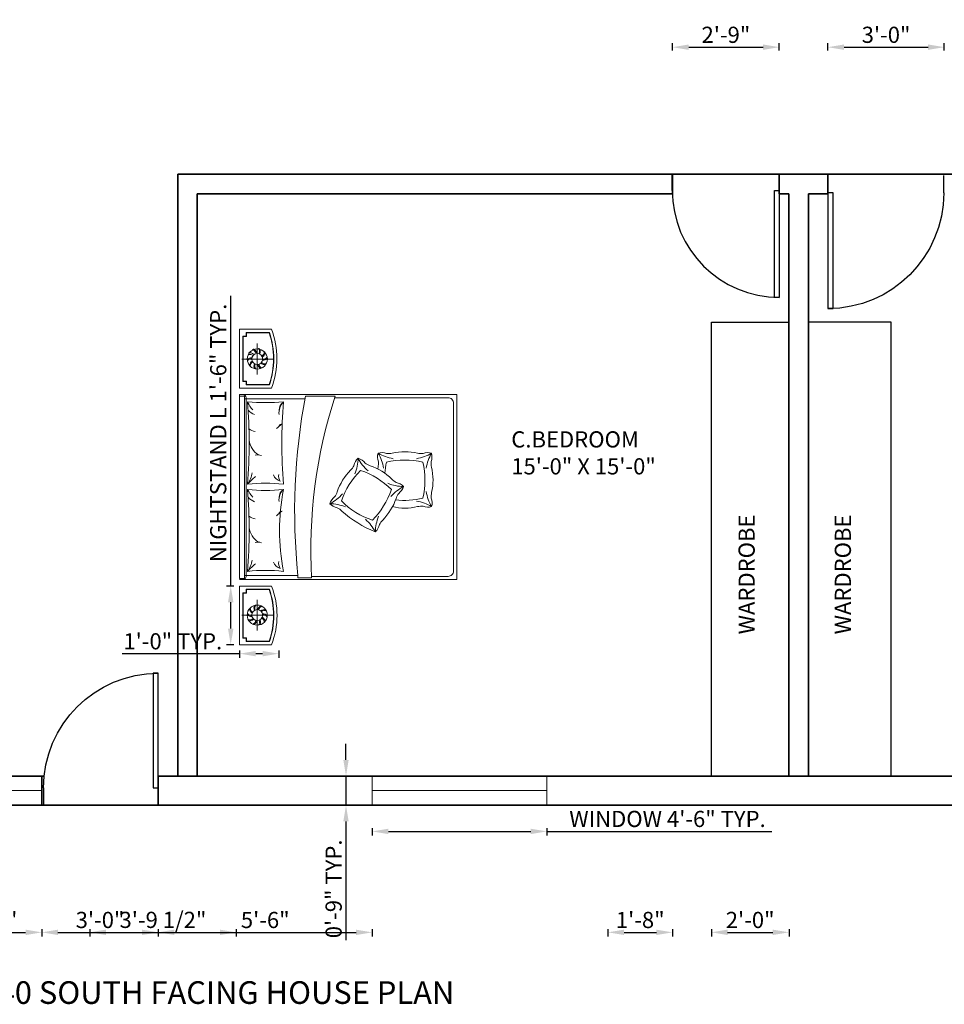
# Model space of a CAD drawing. Units: inches. Extents: x -48 to 817, y -530 to 78.
# Tile 4 of 7: x 266 to 551, y -530 to -225. Entities that reach past the tile are written whole.
import ezdxf

# ---------------------------------------------------------------- set-up
doc = ezdxf.new("R2010")
doc.units = ezdxf.units.IN
for name, color, linetype, lineweight in [('A-ANNO-DIMS', 2, 'Continuous', 18), ('A-AREA-IDEN', 7, 'Continuous', 18), ('A-DOOR', 3, 'Continuous', 25), ('A-FLOR-CASE', 8, 'Continuous', 25), ('A-GLAZ', 4, 'Continuous', 18), ('A-WALL', 7, 'Continuous', 35), ('furn', 8, 'Continuous', 18), ('txt', 7, 'Continuous', 18)]:
    doc.layers.add(name, color=color, linetype=linetype, lineweight=lineweight)
doc.styles.get("Standard").update_dxf_attribs({"font": 'arial.ttf'})
doc.dimstyles.new('ISO-25', dxfattribs={"dimtxt": 5, "dimasz": 5, "dimexe": 1.25, "dimexo": 0.625, "dimtad": 1, "dimlunit": 3, "dimtxsty": 'Standard', "dimcen": 2.5, "dimadec": 0, "dimazin": 0, "dimtfac": 1, "dimtmove": 0, "dimatfit": 3, "dimfxl": 1, "dimfxlon": 1, "dimarcsym": 0})

# ---------------------------------------------------------------- blocks, each defined once
blk = doc.blocks.new('*U2')
for p, q in [((0, 0), (0, -6)), ((40, 0), (40, -6))]:
    blk.add_line(p, q)
blk.add_lwpolyline([(0, 0), (0, 40), (1.75, 40), (1.75, 0)], close=True)
blk.add_arc((0, 0), 40, 0, 90)
blk = doc.blocks.new('BED-DOUBLE')
for p, q in [((0.99, 65.08), (56.21, 65.08)), ((1.28, 65.57), (1.28, 49.06)), ((55.89, 65.57), (55.89, 46.91))]:
    blk.add_line(p, q)
for points in [[(0, 67.12), (0, 0), (57.2, 0), (57.2, 67.12)], [(56.67, 67.12), (56.67, 65.57), (0.33, 65.57), (0.33, 67.12), (57.2, 67.12)]]:
    blk.add_lwpolyline(points)
for points in [[(2.54, 53.57, 0.058596), (2.54, 64.62, 0.036889), (27.85, 64.62, 0.052163), (27.85, 53.57, 0.093111)], [(29.5, 53.57, 0.058596), (29.5, 64.62, 0.036648), (54.99, 64.62, 0.052163), (54.99, 53.57, 0.036967)], [(0.5, 49.06), (1.28, 49.06, -0.072944), (56.67, 46.75), (56.67, 37.58, 0.092568), (0.5, 44.85)]]:
    blk.add_lwpolyline(points, format="xyb", close=True)
for points in [[(0.99, 44.88), (0.99, 2.65, 0.414214), (2.65, 0.99), (54.56, 0.99, 0.414214), (56.21, 2.65), (56.21, 37.74)], [(22.46, 34.35, 0.091296), (23.47, 39.19, 0.091296), (26.52, 35.29, 0.091296)], [(18.37, 26.07, 0.111006), (27.81, 20.2, 0.119549), (33.77, 29.75, 0.107813), (24.35, 35.65)], [(24.3, 35.64, 0.121865), (18.37, 26.07, 0.121865)], [(28.76, 16.41, 0.159461), (30.04, 18.69, -0.076283), (31.05, 20.1, 0.115075), (35.2, 26.76, -0.076283), (36.02, 28.3, 0.159461), (37.5, 30.45)], [(32.66, 31.47, 0.091296), (37.5, 30.45, 0.091296), (33.59, 27.41, 0.091296)], [(19.57, 24.14, 0.091296), (14.72, 25.16, 0.091296), (18.63, 28.19, 0.091296)], [(25.17, 10.45, 0.111006), (36.29, 10.46, 0.119549), (36.29, 21.72, 0.033212), (32.87, 22.24)], [(34.44, 22.59, 0.091296), (39.09, 24.28, 0.091296), (37.38, 19.64, 0.091296)], [(39.09, 7.75, 0.159461), (38.98, 10.35, -0.076283), (39.09, 12.09, 0.115075), (39.09, 19.94, -0.076283), (38.98, 21.68, 0.159461), (39.09, 24.28)], [(29.76, 21.26, 0.091296), (28.76, 16.41, 0.091296), (25.71, 20.31)], [(27.21, 9.44, 0.091296), (22.56, 7.75, 0.091296), (24.27, 12.39, 0.091296)], [(37.38, 12.39, 0.091296), (39.09, 7.75, 0.091296), (34.44, 9.44)]]:
    blk.add_lwpolyline(points, format="xyb")
for centre, radius, start, end in [((0.99, 66.07), 0.992, 180, 270), ((8.41, 73.86), 10.95, 237.5379, 257.5233), ((-5.75, 54.29), 13.24, 36.4935, 51.2792), ((16.81, 58.07), 6.13, 96.6849, 148.3182), ((23.01, 61.56), 4.3, 141.8174, 169.8987), ((28.45, 60.95), 4.63, 130.5354, 160.3558), ((31.33, 57.05), 8.33, 114.6457, 134.1585), ((21.22, 54.29), 13.24, 36.4935, 51.2792), ((35.38, 73.86), 10.95, 237.5379, 257.5233), ((43.78, 58.07), 6.13, 96.6849, 148.3182), ((49.97, 61.56), 4.3, 141.8174, 169.8987), ((55.41, 60.95), 4.63, 130.5354, 160.3558), ((58.29, 57.05), 8.33, 114.6457, 134.1585), ((56.21, 66.07), 0.992, 270, 0), ((8.86, 61.48), 2.75, 335.8927, 16.1192), ((35.82, 61.48), 2.75, 335.8927, 16.1192), ((6.89, 53.32), 3.67, 114.2916, 160.9896), ((4.98, 52.55), 2.51, 76.4823, 128.5563), ((9.99, 45.89), 13.8, 36.2085, 45.0849), ((20.2, 54.04), 0.927, 353.7543, 77.2187), ((24.63, 50.41), 4.52, 44.406, 96.8342), ((25.47, 51.99), 2.86, 33.6349, 90.8456), ((33.85, 53.32), 3.67, 114.2916, 160.9896), ((31.95, 52.55), 2.51, 76.4823, 128.5563), ((36.95, 45.89), 13.8, 36.2085, 45.0849), ((47.16, 54.04), 0.927, 353.7543, 77.2187), ((51.59, 50.41), 4.52, 44.406, 96.8342), ((52.44, 51.99), 2.86, 33.6349, 90.8456), ((17.07, 39.52), 5.74, 315.5854, 333.0343), ((26.3, 36.1), 4.19, 132.4658, 168.7065), ((22.36, 35.3), 4.04, 37.2937, 74.0973), ((29.01, 42.35), 5.74, 233.2983, 250.7472), ((21.6, 20.56), 17.28, 45.1307, 71.3884), ((48.24, 11.46), 36.21, 138.3818, 157.7644), ((37.79, 36.92), 5.74, 225.7718, 243.2208), ((34.51, 27.99), 3.87, 39.4726, 79.6505), ((17.81, 28), 4.19, 222.6522, 258.8929), ((30.83, 7.48), 17.28, 77.0576, 78.7033), ((37.86, 20.61), 3.87, 71.3996, 111.5774), ((14.41, 18.76), 5.74, 45.7718, 63.2208), ((30.61, 35.12), 17.28, 225.1307, 251.3884), ((35.92, 29.93), 5.74, 257.6988, 275.1477), ((39.38, 16.01), 17.28, 166.8711, 193.1289), ((47.91, 16.13), 23.44, 173.1956, 194.0284), ((23.2, 13.33), 5.74, 53.2983, 70.7472), ((30.37, 20.93), 4.79, 218.7754, 250.3571), ((26.6, 8.88), 4.19, 159.3666, 195.6073), ((16.95, 10.85), 5.74, 355.0387, 12.4877), ((23.67, 11.79), 4.19, 254.5791, 290.8198), ((25.68, 2.15), 5.74, 77.6988, 95.1477), ((30.77, 24.6), 17.28, 257.0576, 283.3153), ((36.01, 2.19), 5.74, 85.2252, 102.6741), ((38.07, 12.43), 4.79, 250.7023, 282.284)]:
    blk.add_arc(centre, radius, start, end)
blk = doc.blocks.new('NIGHTSTAND-WITH-LAMP-L')
for p, q in [((9.19, 1.33), (9.19, 10.86)), ((4.42, 6.1), (13.95, 6.1))]:
    blk.add_line(p, q)
blk.add_lwpolyline([(0, 1.65), (0, 11.57), (18.19, 11.57), (18.19, 1.65, -0.181818)], format="xyb", close=True)
for points in [[(2.08, 10.58), (2.08, 9.49), (0.99, 9.49)], [(2.18, 10.58), (2.18, 9.39), (0.99, 9.39)], [(2.08, 10.58), (16.1, 10.58)], [(2.08, 10.48), (16.1, 10.48)], [(16, 10.58), (16, 9.39), (17.19, 9.39)], [(16.1, 10.58), (16.1, 9.49), (17.19, 9.49)]]:
    blk.add_lwpolyline(points)
for points in [[(17.19, 9.49), (17.19, 2.35, -0.167087), (0.99, 2.35), (0.99, 9.49)], [(17.09, 9.49), (17.09, 2.42, -0.165559), (1.09, 2.42), (1.09, 9.49)]]:
    blk.add_lwpolyline(points, format="xyb")
for radius in [3.11, 1.69]:
    blk.add_circle((9.19, 6.1), radius)
for centre, radius, start, end in [((10.78, 7.82), 2, 136.17, 182.4897), ((10.6, 7.9), 1.53, 124.3002, 184.538), ((8.04, 8.15), 2, 208.17, 254.4897), ((7.91, 8), 1.53, 196.3002, 256.538), ((9.46, 8.43), 2, 172.17, 218.4897), ((9.27, 8.39), 1.53, 160.3002, 220.538), ((11.49, 6.56), 2, 100.17, 146.4897), ((11.39, 6.73), 1.53, 88.3002, 148.538), ((11.32, 5.11), 2, 64.17, 110.4897), ((11.34, 5.31), 1.53, 52.3002, 112.538), ((7.03, 6.88), 1.53, 232.3002, 292.538), ((7.05, 7.08), 2, 244.17, 290.4897), ((6.98, 5.47), 1.53, 268.3002, 328.538), ((6.88, 5.64), 2, 280.17, 326.4897), ((7.78, 4.29), 1.53, 304.3002, 4.538), ((7.59, 4.37), 2, 316.17, 2.4897), ((9.11, 3.81), 1.53, 340.3002, 40.538), ((8.91, 3.76), 2, 352.17, 38.4897), ((10.47, 4.2), 1.53, 16.3002, 76.538), ((10.33, 4.05), 2, 28.17, 74.4897)]:
    blk.add_arc(centre, radius, start, end)
blk = doc.blocks.new('NIGHTSTAND-WITH-LAMP-R')
for p, q in [((9, 1.32), (9, 10.86)), ((13.77, 6.09), (4.23, 6.09))]:
    blk.add_line(p, q)
blk.add_lwpolyline([(18.19, 1.65), (18.19, 11.57), (0, 11.57), (0, 1.65, 0.181818)], format="xyb", close=True)
for points in [[(2.08, 10.58), (2.08, 9.49), (0.99, 9.49)], [(2.18, 10.58), (2.18, 9.39), (0.99, 9.39)], [(16.1, 10.58), (2.08, 10.58)], [(16.1, 10.48), (2.08, 10.48)], [(16, 10.58), (16, 9.39), (17.19, 9.39)], [(16.1, 10.58), (16.1, 9.49), (17.19, 9.49)]]:
    blk.add_lwpolyline(points)
for points in [[(0.99, 9.49), (0.99, 2.35, 0.167087), (17.19, 2.35), (17.19, 9.49)], [(1.09, 9.49), (1.09, 2.42, 0.165559), (17.09, 2.42), (17.09, 9.49)]]:
    blk.add_lwpolyline(points, format="xyb")
for radius in [3.11, 1.69]:
    blk.add_circle((9, 6.09), radius)
for centre, radius, start, end in [((7.59, 7.9), 1.53, 355.462, 55.6998), ((7.4, 7.82), 2, 357.5103, 43.83), ((6.85, 5.31), 1.53, 67.462, 127.6998), ((6.87, 5.11), 2, 69.5103, 115.83), ((6.8, 6.72), 1.53, 31.462, 91.6998), ((6.69, 6.55), 2, 33.5103, 79.83), ((8.92, 8.38), 1.53, 319.462, 19.6998), ((8.95, 8.51), 2, 321.5103, 7.83), ((10.51, 8.08), 1.53, 283.462, 343.6998), ((10.37, 8.23), 2, 285.5103, 331.83), ((7.85, 4.04), 2, 105.5103, 151.83), ((7.72, 4.19), 1.53, 103.462, 163.6998), ((9.27, 3.76), 2, 141.5103, 187.83), ((9.08, 3.8), 1.53, 139.462, 199.6998), ((10.59, 4.37), 2, 177.5103, 223.83), ((10.41, 4.29), 1.53, 175.462, 235.6998), ((11.3, 5.63), 2, 213.5103, 259.83), ((11.2, 5.46), 1.53, 211.462, 271.6998), ((11.36, 7.16), 2, 249.5103, 295.83), ((11.38, 6.96), 1.53, 247.462, 307.6998)]:
    blk.add_arc(centre, radius, start, end)
blk = doc.blocks.new('WIN-54IN')
blk.add_line((4.5, 54), (4.5, 0))
blk.add_lwpolyline([(9, 54), (0, 54), (0, 0), (9, 0)], close=True)
blk = doc.blocks.new('*D20')
at = {"layer": 'A-ANNO-DIMS', "color": 0, "lineweight": -2, "transparency": 16777216}
for p, q in [((374.61, -475.39), (374.61, -477.64)), ((379.61, -476.39), (423.61, -476.39)), ((428.61, -475.39), (428.61, -477.64)), ((428.61, -476.39), (498.13, -476.39))]:
    blk.add_line(p, q, dxfattribs=at)
at = {"layer": 'A-ANNO-DIMS', "color": 0, "transparency": 16777216}
for points in [[(379.61, -475.56), (379.61, -477.22), (374.61, -476.39)], [(423.61, -475.56), (423.61, -477.22), (428.61, -476.39)]]:
    blk.add_solid(points, dxfattribs=at)
at = {"layer": 'Defpoints', "color": 0, "transparency": 16777216}
for p in [(374.61, -468.29), (428.61, -468.29), (428.61, -476.39)]:
    blk.add_point(p, dxfattribs=at)
at = {"layer": 'A-ANNO-DIMS', "color": 0, "transparency": 16777216, "insert": (465.87, -473.18), "char_height": 5, "attachment_point": 5}
blk.add_mtext('WINDOW 4\'-6" TYP.', dxfattribs=at)
blk = doc.blocks.new('*D21')
at = {"layer": 'A-ANNO-DIMS', "color": 0, "lineweight": -2, "transparency": 16777216}
for p, q in [((366.51, -454.29), (366.51, -449.29)), ((367.51, -459.29), (365.26, -459.29)), ((366.51, -459.29), (366.51, -468.29)), ((367.51, -468.29), (365.26, -468.29)), ((366.51, -473.29), (366.51, -510.02))]:
    blk.add_line(p, q, dxfattribs=at)
at = {"layer": 'A-ANNO-DIMS', "color": 0, "transparency": 16777216}
for points in [[(365.68, -454.29), (367.34, -454.29), (366.51, -459.29)], [(365.68, -473.29), (367.34, -473.29), (366.51, -468.29)]]:
    blk.add_solid(points, dxfattribs=at)
at = {"layer": 'Defpoints', "color": 0, "transparency": 16777216}
for p in [(374.61, -459.29), (366.51, -468.29), (374.61, -468.29)]:
    blk.add_point(p, dxfattribs=at)
at = {"layer": 'A-ANNO-DIMS', "color": 0, "transparency": 16777216, "insert": (363.33, -494.15), "char_height": 5, "attachment_point": 5, "rotation": 90}
blk.add_mtext('0\'-9" TYP.', dxfattribs=at)
blk = doc.blocks.new('*D34')
at = {"layer": 'A-ANNO-DIMS', "color": 0, "lineweight": -2, "transparency": 16777216}
for p, q in [((330.88, -400.54), (330.88, -310.88)), ((331.88, -400.54), (329.63, -400.54)), ((330.88, -413.72), (330.88, -405.54)), ((331.88, -418.72), (329.63, -418.72))]:
    blk.add_line(p, q, dxfattribs=at)
at = {"layer": 'A-ANNO-DIMS', "color": 0, "transparency": 16777216}
for points in [[(330.05, -405.54), (331.72, -405.54), (330.88, -400.54)], [(330.05, -413.72), (331.72, -413.72), (330.88, -418.72)]]:
    blk.add_solid(points, dxfattribs=at)
at = {"layer": 'Defpoints', "color": 0, "transparency": 16777216}
for p in [(330.88, -400.54), (333.61, -400.54), (333.61, -418.72)]:
    blk.add_point(p, dxfattribs=at)
at = {"layer": 'A-ANNO-DIMS', "color": 0, "transparency": 16777216, "insert": (327.67, -353.21), "char_height": 5, "attachment_point": 5, "rotation": 90}
blk.add_mtext('NIGHTSTAND L 1\'-6" TYP.', dxfattribs=at)
blk = doc.blocks.new('*D35')
at = {"layer": 'A-ANNO-DIMS', "color": 0, "lineweight": -2, "transparency": 16777216}
for p, q in [((333.61, -421.45), (297.36, -421.45)), ((333.61, -420.45), (333.61, -422.7)), ((340.74, -421.45), (338.61, -421.45)), ((345.74, -420.45), (345.74, -422.7))]:
    blk.add_line(p, q, dxfattribs=at)
at = {"layer": 'A-ANNO-DIMS', "color": 0, "transparency": 16777216}
for points in [[(338.61, -420.62), (338.61, -422.28), (333.61, -421.45)], [(340.74, -420.62), (340.74, -422.28), (345.74, -421.45)]]:
    blk.add_solid(points, dxfattribs=at)
at = {"layer": 'Defpoints', "color": 0, "transparency": 16777216}
for p in [(333.61, -418.72), (345.74, -418.72), (333.61, -421.45)]:
    blk.add_point(p, dxfattribs=at)
at = {"layer": 'A-ANNO-DIMS', "color": 0, "transparency": 16777216, "insert": (312.98, -418.27), "char_height": 5, "attachment_point": 5}
blk.add_mtext('1\'-0" TYP.', dxfattribs=at)
blk = doc.blocks.new('*D45')
at = {"layer": 'A-ANNO-DIMS', "color": 0, "lineweight": -2, "transparency": 16777216}
for p, q in [((272.5, -506.59), (272.5, -508.84)), ((277.5, -507.59), (303.5, -507.59)), ((308.5, -506.59), (308.5, -508.84))]:
    blk.add_line(p, q, dxfattribs=at)
at = {"layer": 'A-ANNO-DIMS', "color": 0, "transparency": 16777216}
for points in [[(277.5, -506.76), (277.5, -508.42), (272.5, -507.59)], [(303.5, -506.76), (303.5, -508.42), (308.5, -507.59)]]:
    blk.add_solid(points, dxfattribs=at)
at = {"layer": 'Defpoints', "color": 0, "transparency": 16777216}
for p in [(272.5, -468.28), (308.5, -468.28), (308.5, -507.59)]:
    blk.add_point(p, dxfattribs=at)
at = {"layer": 'A-ANNO-DIMS', "color": 0, "transparency": 16777216, "insert": (290.5, -504.41), "char_height": 5, "attachment_point": 5}
blk.add_mtext('3\'-0"', dxfattribs=at)
blk = doc.blocks.new('*D57')
at = {"layer": 'A-ANNO-DIMS', "color": 0, "lineweight": -2, "transparency": 16777216}
for p, q in [((308.5, -506.59), (308.5, -508.84)), ((313.5, -507.59), (369.61, -507.59)), ((374.61, -506.59), (374.61, -508.84))]:
    blk.add_line(p, q, dxfattribs=at)
at = {"layer": 'A-ANNO-DIMS', "color": 0, "transparency": 16777216}
for points in [[(313.5, -506.76), (313.5, -508.42), (308.5, -507.59)], [(369.61, -506.76), (369.61, -508.42), (374.61, -507.59)]]:
    blk.add_solid(points, dxfattribs=at)
at = {"layer": 'Defpoints', "color": 0, "transparency": 16777216}
for p in [(308.5, -468.28), (374.61, -468.29), (374.61, -507.59)]:
    blk.add_point(p, dxfattribs=at)
at = {"layer": 'A-ANNO-DIMS', "color": 0, "transparency": 16777216, "insert": (341.55, -504.41), "char_height": 5, "attachment_point": 5}
blk.add_mtext('5\'-6"', dxfattribs=at)
blk = doc.blocks.new('*D62')
at = {"layer": 'A-ANNO-DIMS', "color": 0, "lineweight": -2, "transparency": 16777216}
for p, q in [((-35.87, -239.28), (-38.12, -239.28)), ((-36.87, -244.28), (-36.87, -264.28)), ((-35.87, -269.28), (-38.12, -269.28))]:
    blk.add_line(p, q, dxfattribs=at)
at = {"layer": 'A-ANNO-DIMS', "color": 0, "transparency": 16777216}
for points in [[(-37.71, -244.28), (-36.04, -244.28), (-36.87, -239.28)], [(-37.71, -264.28), (-36.04, -264.28), (-36.87, -269.28)]]:
    blk.add_solid(points, dxfattribs=at)
at = {"layer": 'Defpoints', "color": 0, "transparency": 16777216}
for p in [(593.43, -239.28), (-36.87, -269.28), (593.43, -269.28)]:
    blk.add_point(p, dxfattribs=at)
at = {"layer": 'A-ANNO-DIMS', "color": 0, "transparency": 16777216, "insert": (-40.05, -254.28), "char_height": 5, "attachment_point": 5, "rotation": 90}
blk.add_mtext('2\'-6"', dxfattribs=at)
blk = doc.blocks.new('*D63')
at = {"layer": 'A-ANNO-DIMS', "color": 0, "lineweight": -2, "transparency": 16777216}
for p, q in [((467.43, -234.98), (467.43, -232.73)), ((472.43, -233.98), (495.43, -233.98)), ((500.43, -234.98), (500.43, -232.73))]:
    blk.add_line(p, q, dxfattribs=at)
at = {"layer": 'A-ANNO-DIMS', "color": 0, "transparency": 16777216}
for points in [[(472.43, -233.14), (472.43, -234.81), (467.43, -233.98)], [(495.43, -233.14), (495.43, -234.81), (500.43, -233.98)]]:
    blk.add_solid(points, dxfattribs=at)
at = {"layer": 'Defpoints', "color": 0, "transparency": 16777216}
for p in [(500.43, -233.98), (467.43, -273.28), (500.43, -273.28)]:
    blk.add_point(p, dxfattribs=at)
at = {"layer": 'A-ANNO-DIMS', "color": 0, "transparency": 16777216, "insert": (483.93, -230.8), "char_height": 5, "attachment_point": 5}
blk.add_mtext('2\'-9"', dxfattribs=at)
blk = doc.blocks.new('*D64')
at = {"layer": 'A-ANNO-DIMS', "color": 0, "lineweight": -2, "transparency": 16777216}
for p, q in [((515.43, -234.98), (515.43, -232.73)), ((520.43, -233.98), (546.43, -233.98)), ((551.43, -234.98), (551.43, -232.73))]:
    blk.add_line(p, q, dxfattribs=at)
at = {"layer": 'A-ANNO-DIMS', "color": 0, "transparency": 16777216}
for points in [[(520.43, -233.14), (520.43, -234.81), (515.43, -233.98)], [(546.43, -233.14), (546.43, -234.81), (551.43, -233.98)]]:
    blk.add_solid(points, dxfattribs=at)
at = {"layer": 'Defpoints', "color": 0, "transparency": 16777216}
for p in [(551.43, -233.98), (515.43, -273.28), (551.43, -273.28)]:
    blk.add_point(p, dxfattribs=at)
at = {"layer": 'A-ANNO-DIMS', "color": 0, "transparency": 16777216, "insert": (533.43, -230.8), "char_height": 5, "attachment_point": 5}
blk.add_mtext('3\'-0"', dxfattribs=at)
blk = doc.blocks.new('*D65')
at = {"layer": 'A-ANNO-DIMS', "color": 0, "lineweight": -2, "transparency": 16777216}
for p, q in [((811.62, -384.28), (813.87, -384.28)), ((812.62, -389.28), (812.62, -409.4)), ((811.62, -414.4), (813.87, -414.4))]:
    blk.add_line(p, q, dxfattribs=at)
at = {"layer": 'A-ANNO-DIMS', "color": 0, "transparency": 16777216}
for points in [[(811.79, -389.28), (813.45, -389.28), (812.62, -384.28)], [(811.79, -409.4), (813.45, -409.4), (812.62, -414.4)]]:
    blk.add_solid(points, dxfattribs=at)
at = {"layer": 'Defpoints', "color": 0, "transparency": 16777216}
for p in [(161.43, -384.28), (161.43, -414.4), (812.62, -414.4)]:
    blk.add_point(p, dxfattribs=at)
at = {"layer": 'A-ANNO-DIMS', "color": 0, "transparency": 16777216, "insert": (809.44, -399.34), "char_height": 5, "attachment_point": 5, "rotation": 90}
blk.add_mtext('2\'-6"', dxfattribs=at)
blk = doc.blocks.new('*D66')
at = {"layer": 'A-ANNO-DIMS', "color": 0, "lineweight": -2, "transparency": 16777216}
for p, q in [((811.62, -414.4), (813.87, -414.4)), ((812.62, -419.4), (812.62, -454.28)), ((811.62, -459.28), (813.87, -459.28))]:
    blk.add_line(p, q, dxfattribs=at)
at = {"layer": 'A-ANNO-DIMS', "color": 0, "transparency": 16777216}
for points in [[(811.79, -419.4), (813.45, -419.4), (812.62, -414.4)], [(811.79, -454.28), (813.45, -454.28), (812.62, -459.28)]]:
    blk.add_solid(points, dxfattribs=at)
at = {"layer": 'Defpoints', "color": 0, "transparency": 16777216}
for p in [(161.43, -414.4), (161.43, -459.28), (812.62, -459.28)]:
    blk.add_point(p, dxfattribs=at)
at = {"layer": 'A-ANNO-DIMS', "color": 0, "transparency": 16777216, "insert": (809.44, -436.84), "char_height": 5, "attachment_point": 5, "rotation": 90}
blk.add_mtext('3\'-9"', dxfattribs=at)
blk = doc.blocks.new('*D69')
at = {"layer": 'A-ANNO-DIMS', "color": 0, "lineweight": -2, "transparency": 16777216}
for p, q in [((479.43, -506.59), (479.43, -508.84)), ((484.43, -507.59), (498.43, -507.59)), ((503.43, -506.59), (503.43, -508.84))]:
    blk.add_line(p, q, dxfattribs=at)
at = {"layer": 'A-ANNO-DIMS', "color": 0, "transparency": 16777216}
for points in [[(484.43, -506.76), (484.43, -508.42), (479.43, -507.59)], [(498.43, -506.76), (498.43, -508.42), (503.43, -507.59)]]:
    blk.add_solid(points, dxfattribs=at)
at = {"layer": 'Defpoints', "color": 0, "transparency": 16777216}
for p in [(479.43, -459.28), (503.43, -459.28), (503.43, -507.59)]:
    blk.add_point(p, dxfattribs=at)
at = {"layer": 'A-ANNO-DIMS', "color": 0, "transparency": 16777216, "insert": (491.43, -504.41), "char_height": 5, "attachment_point": 5}
blk.add_mtext('2\'-0"', dxfattribs=at)
blk = doc.blocks.new('*D70')
at = {"layer": 'A-ANNO-DIMS', "color": 0, "lineweight": -2, "transparency": 16777216}
for p, q in [((-35.87, -319.02), (-38.12, -319.02)), ((-36.87, -324.02), (-36.87, -454.28)), ((-35.87, -459.28), (-38.12, -459.28))]:
    blk.add_line(p, q, dxfattribs=at)
at = {"layer": 'A-ANNO-DIMS', "color": 0, "transparency": 16777216}
for points in [[(-37.71, -324.02), (-36.04, -324.02), (-36.87, -319.02)], [(-37.71, -454.28), (-36.04, -454.28), (-36.87, -459.28)]]:
    blk.add_solid(points, dxfattribs=at)
at = {"layer": 'Defpoints', "color": 0, "transparency": 16777216}
for p in [(479.43, -319.02), (-36.87, -459.28), (479.43, -459.28)]:
    blk.add_point(p, dxfattribs=at)
at = {"layer": 'A-ANNO-DIMS', "color": 0, "transparency": 16777216, "insert": (-40.08, -389.15), "char_height": 5, "attachment_point": 5, "rotation": 90}
blk.add_mtext('11\'-8 1/2"', dxfattribs=at)
blk = doc.blocks.new('*D75')
at = {"layer": 'A-ANNO-DIMS', "color": 0, "lineweight": -2, "transparency": 16777216}
for p, q in [((287.29, -506.59), (287.29, -508.84)), ((292.29, -507.59), (327.6, -507.59)), ((332.6, -506.59), (332.6, -508.84))]:
    blk.add_line(p, q, dxfattribs=at)
at = {"layer": 'A-ANNO-DIMS', "color": 0, "transparency": 16777216}
for points in [[(292.29, -506.76), (292.29, -508.42), (287.29, -507.59)], [(327.6, -506.76), (327.6, -508.42), (332.6, -507.59)]]:
    blk.add_solid(points, dxfattribs=at)
at = {"layer": 'Defpoints', "color": 0, "transparency": 16777216}
for p in [(287.29, -130.76), (332.6, -130.76), (332.6, -507.59)]:
    blk.add_point(p, dxfattribs=at)
at = {"layer": 'A-ANNO-DIMS', "color": 0, "transparency": 16777216, "insert": (309.94, -504.38), "char_height": 5, "attachment_point": 5}
blk.add_mtext('3\'-9 1/2"', dxfattribs=at)
blk = doc.blocks.new('*D79')
at = {"layer": 'A-ANNO-DIMS', "color": 0, "lineweight": -2, "transparency": 16777216}
for p, q in [((447.47, -506.59), (447.47, -508.84)), ((452.47, -507.59), (462.43, -507.59)), ((467.43, -506.59), (467.43, -508.84))]:
    blk.add_line(p, q, dxfattribs=at)
at = {"layer": 'A-ANNO-DIMS', "color": 0, "transparency": 16777216}
for points in [[(452.47, -506.76), (452.47, -508.42), (447.47, -507.59)], [(462.43, -506.76), (462.43, -508.42), (467.43, -507.59)]]:
    blk.add_solid(points, dxfattribs=at)
at = {"layer": 'Defpoints', "color": 0, "transparency": 16777216}
for p in [(447.47, -166.39), (467.43, -166.39), (467.43, -507.59)]:
    blk.add_point(p, dxfattribs=at)
at = {"layer": 'A-ANNO-DIMS', "color": 0, "transparency": 16777216, "insert": (457.45, -504.41), "char_height": 5, "attachment_point": 5}
blk.add_mtext('1\'-8"', dxfattribs=at)
blk = doc.blocks.new('*D84')
at = {"layer": 'A-ANNO-DIMS', "color": 0, "lineweight": -2, "transparency": 16777216}
for p, q in [((-35.87, -425.28), (-38.12, -425.28)), ((-36.87, -450.28), (-36.87, -430.28)), ((-35.87, -455.28), (-38.12, -455.28))]:
    blk.add_line(p, q, dxfattribs=at)
at = {"layer": 'A-ANNO-DIMS', "color": 0, "transparency": 16777216}
for points in [[(-37.71, -430.28), (-36.04, -430.28), (-36.87, -425.28)], [(-37.71, -450.28), (-36.04, -450.28), (-36.87, -455.28)]]:
    blk.add_solid(points, dxfattribs=at)
at = {"layer": 'Defpoints', "color": 0, "transparency": 16777216}
for p in [(-36.87, -425.28), (623.43, -425.28), (623.43, -455.28)]:
    blk.add_point(p, dxfattribs=at)
at = {"layer": 'A-ANNO-DIMS', "color": 0, "transparency": 16777216, "insert": (-40.05, -440.28), "char_height": 5, "attachment_point": 5, "rotation": 90}
blk.add_mtext('2\'-6"', dxfattribs=at)
blk = doc.blocks.new('*D85')
at = {"layer": 'A-ANNO-DIMS', "color": 0, "lineweight": -2, "transparency": 16777216}
for p, q in [((238.5, -506.59), (238.5, -508.84)), ((243.5, -507.59), (267.5, -507.59)), ((272.5, -506.59), (272.5, -508.84))]:
    blk.add_line(p, q, dxfattribs=at)
at = {"layer": 'A-ANNO-DIMS', "color": 0, "transparency": 16777216}
for points in [[(243.5, -506.76), (243.5, -508.42), (238.5, -507.59)], [(267.5, -506.76), (267.5, -508.42), (272.5, -507.59)]]:
    blk.add_solid(points, dxfattribs=at)
at = {"layer": 'Defpoints', "color": 0, "transparency": 16777216}
for p in [(238.5, -468.28), (272.5, -468.28), (272.5, -507.59)]:
    blk.add_point(p, dxfattribs=at)
at = {"layer": 'A-ANNO-DIMS', "color": 0, "transparency": 16777216, "insert": (255.5, -504.41), "char_height": 5, "attachment_point": 5}
blk.add_mtext('2\'-10"', dxfattribs=at)

msp = doc.modelspace()

# ---------------------------------------------------------------- linework, layer by layer
at = {"layer": 'A-FLOR-CASE'}
for p, q in [((479.427, -459.275), (479.427, -319.021)), ((479.427, -319.021), (503.427, -319.021)), ((534.963, -319.021), (509.427, -319.021)), ((534.963, -459.275), (534.963, -319.021))]:
    msp.add_line(p, q, dxfattribs=at)
at = {"layer": 'A-GLAZ'}
msp.add_line((272.498, -463.775), (238.498, -463.775), dxfattribs=at)
at = {"layer": 'A-WALL'}
for p, q in [((314.498, -273.275), (503.427, -273.275)), ((314.498, -279.275), (314.498, -273.275)), ((467.427, -273.275), (467.427, -279.275)), ((500.427, -279.275), (500.427, -273.275)), ((509.427, -273.275), (503.427, -273.275)), ((509.427, -273.275), (713.427, -273.275)), ((515.427, -279.275), (515.427, -273.275)), ((314.498, -459.275), (314.498, -279.275)), ((320.498, -459.275), (320.498, -279.275)), ((320.498, -279.275), (463.461, -279.275)), ((467.427, -279.275), (463.461, -279.275)), ((503.427, -279.275), (500.427, -279.275)), ((503.427, -459.275), (503.427, -279.275)), ((509.427, -459.275), (509.427, -279.275)), ((509.427, -279.275), (515.427, -279.275)), ((273.233, -459.275), (11.427, -459.275)), ((272.498, -459.275), (272.498, -468.275)), ((308.498, -459.275), (308.498, -468.275)), ((623.427, -459.275), (308.498, -459.275)), ((722.427, -468.275), (2.427, -468.275))]:
    msp.add_line(p, q, dxfattribs=at)

# ---------------------------------------------------------------- block references
at = {"layer": 'A-DOOR', "rotation": 180}
for p, xscale, yscale, zscale in [((500.427, -278.238), 0.8270996701492702, 0.8270996701492702, 0.8270996701492702), ((515.475, -279.033), -0.8942941617954382, 0.8942941617954382, 0.8942941617954382)]:
    msp.add_blockref('*U2', p, dxfattribs=dict(at, xscale=xscale, yscale=yscale, zscale=zscale))
at = {"layer": 'A-DOOR', "xscale": -0.8864188079995388, "yscale": 0.8864188079995388, "zscale": 0.8864188079995388}
msp.add_blockref('*U2', (308.498, -462.957), dxfattribs=at)
at = {"layer": 'A-GLAZ', "rotation": 269.9999999999998}
msp.add_blockref('WIN-54IN', (374.609, -459.289), dxfattribs=at)
at = {"layer": 'furn'}
for name, p, rotation in [('NIGHTSTAND-WITH-LAMP-R', (345.182, -339.368), 90.00000000000115), ('BED-DOUBLE', (400.729, -398.554), 89.99999999999991), ('NIGHTSTAND-WITH-LAMP-L', (345.185, -418.723), 90.00000000000101)]:
    msp.add_blockref(name, p, dxfattribs=dict(at, rotation=rotation))

# ---------------------------------------------------------------- texts
at = {"layer": 'A-AREA-IDEN', "insert": (417.593, -352.71), "char_height": 5, "attachment_point": 1}
msp.add_mtext_dynamic_manual_height_columns('C.BEDROOM\\P15\'-0" X 15\'-0"', width=48.14676, gutter_width=12.5, heights=[0], dxfattribs=at)
at = {"layer": 'txt', "char_height": 5, "attachment_point": 1, "rotation": 90}
for insert in [(487.828, -415.486), (517.571, -415.486)]:
    msp.add_mtext_dynamic_manual_height_columns('WARDROBE', width=73.16203, gutter_width=12.5, heights=[0], dxfattribs=dict(at, insert=insert))
at = {"layer": 'txt', "insert": (242.785, -522.709), "char_height": 7, "attachment_point": 1}
msp.add_mtext_dynamic_manual_height_columns('60X40 SOUTH FACING HOUSE PLAN', width=437.74312, gutter_width=12.5, heights=[0], dxfattribs=at)

# ---------------------------------------------------------------- dimensions: what is measured, and where the dimension line sits
at = {"layer": 'A-ANNO-DIMS'}
for base, p1, p2, picture, middle in [((332.597, -507.589), (287.287, -130.757), (332.597, -130.757), '*D75', (309.942, -504.377)), ((467.427, -507.589), (447.473, -166.393), (467.427, -166.393), '*D79', (457.45, -504.411)), ((500.427, -233.975), (467.427, -273.275), (500.427, -273.275), '*D63', (483.927, -230.798)), ((551.427, -233.975), (515.427, -273.275), (551.427, -273.275), '*D64', (533.427, -230.796)), ((503.427, -507.589), (479.427, -459.275), (503.427, -459.275), '*D69', (491.427, -504.411)), ((272.498, -507.589), (238.498, -468.275), (272.498, -468.275), '*D85', (255.498, -504.411)), ((308.498, -507.589), (272.498, -468.275), (308.498, -468.275), '*D45', (290.498, -504.409)), ((374.609, -507.589), (308.498, -468.275), (374.609, -468.289), '*D57', (341.554, -504.411))]:
    dim = msp.add_linear_dim(base=base, p1=p1, p2=p2, dimstyle='ISO-25', override={"dimdec": 1, "dimlfac": 1, "dimrnd": 0, "dimzin": 1, "dimdsep": 46, "dimlunit": 4, "dimfrac": 2}, dxfattribs=at)
    dim.commit()
    dim.dimension.update_dxf_attribs({"geometry": picture, "text_midpoint": middle})
for base, p1, p2, picture, middle in [((-36.873, -269.275), (593.427, -239.275), (593.427, -269.275), '*D62', (-40.051, -254.275)), ((-36.873, -459.275), (479.427, -319.021), (479.427, -459.275), '*D70', (-40.083, -389.148)), ((812.622, -414.396), (161.427, -384.275), (161.427, -414.396), '*D65', (809.444, -399.336)), ((812.622, -459.275), (161.427, -414.396), (161.427, -459.275), '*D66', (809.442, -436.836)), ((-36.873, -425.275), (623.427, -455.275), (623.427, -425.275), '*D84', (-40.051, -440.275))]:
    dim = msp.add_linear_dim(base=base, p1=p1, p2=p2, angle=90, dimstyle='ISO-25', override={"dimdec": 1, "dimlfac": 1, "dimrnd": 0, "dimzin": 1, "dimdsep": 46, "dimlunit": 4, "dimfrac": 2}, dxfattribs=at)
    dim.commit()
    dim.dimension.update_dxf_attribs({"geometry": picture, "text_midpoint": middle})
for base, p1, p2, angle, text, picture, middle in [((330.885, -400.538), (333.613, -418.723), (333.613, -400.538), 90, 'NIGHTSTAND L <> TYP.', '*D34', (327.675, -353.211)), ((333.613, -421.451), (345.736, -418.723), (333.613, -418.723), 180, '<> TYP.', '*D35', (312.984, -418.273)), ((366.509, -468.289), (374.609, -459.289), (374.609, -468.289), 270, '<> TYP.', '*D21', (363.331, -494.153))]:
    dim = msp.add_linear_dim(base=base, p1=p1, p2=p2, angle=angle, text=text, dimstyle='ISO-25', override={"dimdec": 1, "dimlfac": 1, "dimrnd": 0, "dimzin": 1, "dimdsep": 46, "dimlunit": 4, "dimfrac": 2}, dxfattribs=at)
    dim.commit()
    dim.dimension.update_dxf_attribs({"geometry": picture, "text_midpoint": middle})
dim = msp.add_linear_dim(base=(428.609, -476.389), p1=(374.609, -468.289), p2=(428.609, -468.289), text='WINDOW <> TYP.', dimstyle='ISO-25', override={"dimdec": 1, "dimlfac": 1, "dimrnd": 0, "dimzin": 1, "dimdsep": 46, "dimlunit": 4, "dimfrac": 2}, dxfattribs=at)
dim.commit()
dim.dimension.update_dxf_attribs({"geometry": '*D20', "text_midpoint": (465.869, -473.177)})

doc.saveas('drawing.dxf')
